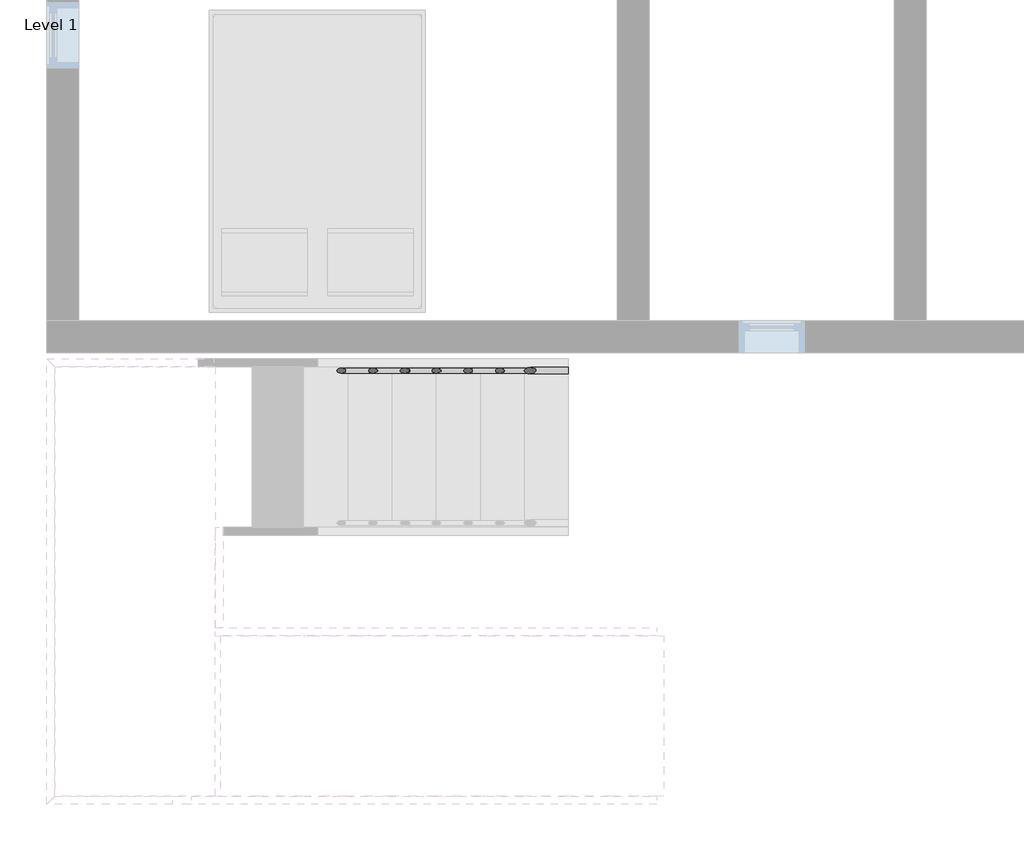
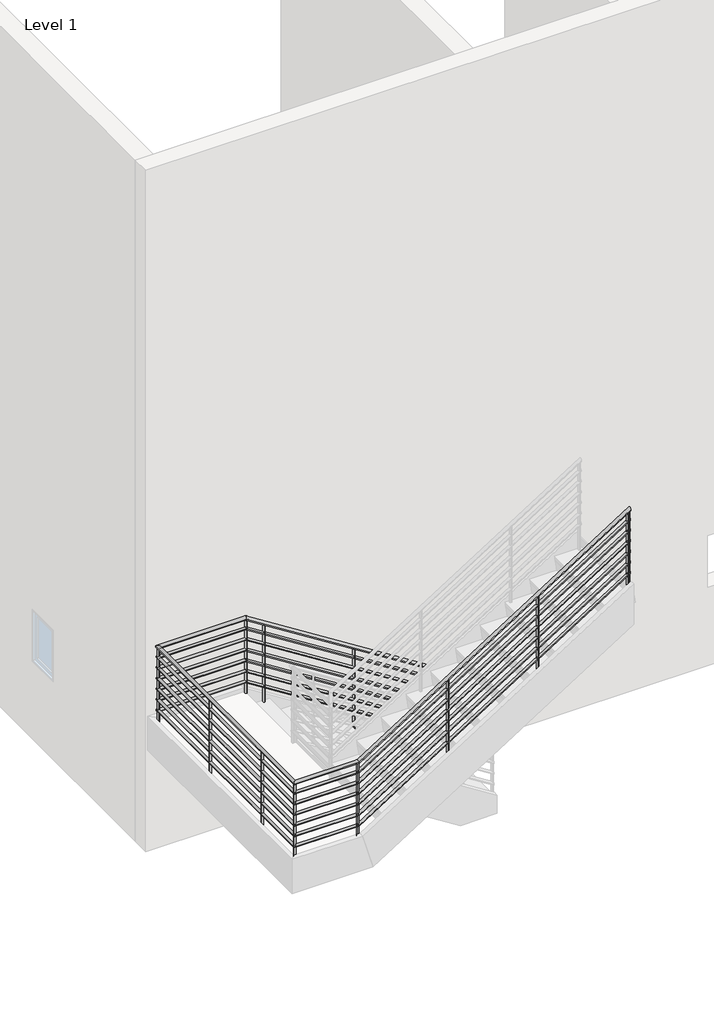
# One storey, part 2 of 4: 1 railing.
"""IFC4 building model written with IfcOpenShell, lengths in millimetres."""

from ifc_helpers import new_model, si_unit, point, frame, frame_2d, origin, place, context, project, spatial, circle_curve, ellipse_curve, trimmed, segment, composite_curve, outline, extrude, element, save
from ifc_brep_helpers import plane_surface, cylinder_surface, advanced_brep

model = new_model("IFC4")

# Units and contexts
model_context = context("Model", 3, world=origin())
ifc_project = project(units=[si_unit("LENGTHUNIT", "METRE", prefix="MILLI")], contexts=[model_context])

# Site, building, storey
site = spatial("IfcSite", under=ifc_project)
building = spatial("IfcBuilding", under=site)
storey = spatial("IfcBuildingStorey", under=building, Name="Level 1", Elevation=0.0)

# Railing
placement = place(None, origin())
element("IfcRailing", 1, ObjectType="900mm Pipe", at=placement, inside=storey, context=model_context, shape_type="SolidModel", body=[
    advanced_brep(
    [(-8274.8492596, 6241.5562283, 1050.2491997), (-8274.8492596, 6201.5562283, 1050.2491997), (-10480.6427126, 6241.5562283, 2445.2173913), (-10480.6427126, 6201.5562283, 2445.2173913), (-11469.4750408, 6241.5562283, 2445.2173913), (-11429.4750408, 6201.5562283, 2445.2173913), (-11469.4750408, 3575.930447, 2445.2173913), (-11429.4750408, 3615.930447, 2445.2173913), (-10744.0558066, 3575.930447, 2445.2173913), (-10744.0558066, 3615.930447, 2445.2173913), (-7724.8492596, 3575.930447, 4354.5970258), (-7724.8492596, 3615.930447, 4354.5970258)],
    [
        (0, 1, ellipse_curve(frame((-8274.8492596, 6221.5562283, 1050.2491997), z_axis=(1.0, 0.0, 0.0), x_axis=(0.0, 0.0, -1.0)), 23.6638438, 20.0)),
        (1, 0, ellipse_curve(frame((-8274.8492596, 6221.5562283, 1050.2491997), z_axis=(1.0, 0.0, 0.0), x_axis=(0.0, 0.0, -1.0)), 23.6638438, 20.0)),
        (0, 2),
        (2, 3, ellipse_curve(frame((-10480.6427126, 6221.5562283, 2445.2173913), z_axis=(0.9605132043335073, 0.0, -0.2782344053149758), x_axis=(-0.2782344053149764, 0.0, -0.9605132043335071)), 20.822202, 20.0)),
        (3, 1),
        (3, 2, ellipse_curve(frame((-10480.6427126, 6221.5562283, 2445.2173913), z_axis=(0.9605132043335073, 0.0, -0.2782344053149758), x_axis=(-0.2782344053149764, 0.0, -0.9605132043335071)), 20.822202, 20.0)),
        (2, 4),
        (4, 5, ellipse_curve(frame((-11449.4750408, 6221.5562283, 2445.2173913), z_axis=(0.7071067811865516, 0.7071067811865435, 0.0), x_axis=(0.7071067811865436, -0.7071067811865516, 0.0)), 28.2842712, 20.0)),
        (5, 3),
        (5, 4, ellipse_curve(frame((-11449.4750408, 6221.5562283, 2445.2173913), z_axis=(0.7071067811865516, 0.7071067811865435, 0.0), x_axis=(0.7071067811865436, -0.7071067811865516, 0.0)), 28.2842712, 20.0)),
        (4, 6),
        (6, 7, ellipse_curve(frame((-11449.4750408, 3595.930447, 2445.2173913), z_axis=(-0.7071067811865436, 0.7071067811865513, 0.0), x_axis=(0.7071067811865512, 0.7071067811865438, 0.0)), 28.2842712, 20.0)),
        (7, 5),
        (7, 6, ellipse_curve(frame((-11449.4750408, 3595.930447, 2445.2173913), z_axis=(-0.7071067811865436, 0.7071067811865513, 0.0), x_axis=(0.7071067811865512, 0.7071067811865438, 0.0)), 28.2842712, 20.0)),
        (6, 8),
        (8, 9, ellipse_curve(frame((-10744.0558066, 3595.930447, 2445.2173913), z_axis=(-0.9605132043335073, 0.0, -0.2782344053149758), x_axis=(-0.2782344053149755, 0.0, 0.9605132043335073)), 20.822202, 20.0)),
        (9, 7),
        (9, 8, ellipse_curve(frame((-10744.0558066, 3595.930447, 2445.2173913), z_axis=(-0.9605132043335073, 0.0, -0.2782344053149758), x_axis=(-0.2782344053149755, 0.0, 0.9605132043335073)), 20.822202, 20.0)),
        (10, 11, ellipse_curve(frame((-7724.8492596, 3595.930447, 4354.5970258), z_axis=(1.0, 0.0, 0.0), x_axis=(0.0, 0.0, -1.0)), 23.6638438, 20.0)),
        (11, 10, ellipse_curve(frame((-7724.8492596, 3595.930447, 4354.5970258), z_axis=(1.0, 0.0, 0.0), x_axis=(0.0, 0.0, -1.0)), 23.6638438, 20.0)),
        (8, 10),
        (11, 9),
    ],
    [
        plane_surface(frame((-8274.8492596, 6221.5562283, 1073.9130435), z_axis=(1.0, 0.0, 0.0), x_axis=(0.0, -1.0, 0.0))),
        cylinder_surface(frame((-8285.5391724, 6221.5562283, 1057.0096189), z_axis=(0.8451712313980436, 0.0, -0.5344956404098303), x_axis=(0.0, -1.0, 0.0)), 20.0),
        cylinder_surface(frame((-10474.8492596, 6221.5562283, 2445.2173913), z_axis=(1.0, 0.0, 0.0), x_axis=(0.0, -1.0, 0.0)), 20.0),
        cylinder_surface(frame((-11449.4750408, 6221.5562283, 2445.2173913), z_axis=(0.0, 1.0, 0.0), x_axis=(1.0, 0.0, 0.0)), 20.0),
        cylinder_surface(frame((-11449.4750408, 3595.930447, 2445.2173913), z_axis=(-1.0, 0.0, 0.0), x_axis=(0.0, 1.0, 0.0)), 20.0),
        plane_surface(frame((-7724.8492596, 3595.930447, 4378.2608696), z_axis=(1.0, 0.0, 0.0), x_axis=(0.0, 1.0, 0.0))),
        cylinder_surface(frame((-10739.1593468, 3595.930447, 2448.3139667), z_axis=(-0.8451712313980436, 0.0, -0.5344956404098303), x_axis=(0.0, 1.0, 0.0)), 20.0),
    ],
    [
        (0, [[1, 2]]),
        (1, [[-1, 3, 4, 5]]),
        (1, [[-2, -5, 6, -3]]),
        (2, [[-4, 7, 8, 9]]),
        (2, [[-6, -9, 10, -7]]),
        (3, [[-8, 11, 12, 13]]),
        (3, [[-10, -13, 14, -11]]),
        (4, [[-12, 15, 16, 17]]),
        (4, [[-14, -17, 18, -15]]),
        (5, [[19, 20]]),
        (6, [[-16, 21, -20, 22]]),
        (6, [[-18, -22, -19, -21]]),
    ],
),
    advanced_brep(
    [(-8274.8492596, 6206.5562283, 931.1651606), (-8274.8492596, 6236.5562283, 931.1651606), (-10479.1943493, 6206.5562283, 2325.2173913), (-10479.1943493, 6236.5562283, 2325.2173913), (-11434.4750408, 6206.5562283, 2325.2173913), (-11464.4750408, 6236.5562283, 2325.2173913), (-11434.4750408, 3610.930447, 2325.2173913), (-11464.4750408, 3580.930447, 2325.2173913), (-10745.5041698, 3610.930447, 2325.2173913), (-10745.5041698, 3580.930447, 2325.2173913), (-7724.8492596, 3610.930447, 4235.5129867), (-7724.8492596, 3580.930447, 4235.5129867)],
    [
        (0, 1, ellipse_curve(frame((-8274.8492596, 6221.5562283, 931.1651606), z_axis=(1.0, 0.0, 0.0), x_axis=(0.0, 0.0, -1.0)), 17.7478828, 15.0)),
        (1, 0, ellipse_curve(frame((-8274.8492596, 6221.5562283, 931.1651606), z_axis=(1.0, 0.0, 0.0), x_axis=(0.0, 0.0, -1.0)), 17.7478828, 15.0)),
        (0, 2),
        (2, 3, ellipse_curve(frame((-10479.1943493, 6221.5562283, 2325.2173913), z_axis=(0.9605132043335073, 0.0, -0.2782344053149758), x_axis=(-0.2782344053149764, 0.0, -0.9605132043335071)), 15.6166515, 15.0)),
        (3, 1),
        (3, 2, ellipse_curve(frame((-10479.1943493, 6221.5562283, 2325.2173913), z_axis=(0.9605132043335073, 0.0, -0.2782344053149758), x_axis=(-0.2782344053149764, 0.0, -0.9605132043335071)), 15.6166515, 15.0)),
        (2, 4),
        (4, 5, ellipse_curve(frame((-11449.4750408, 6221.5562283, 2325.2173913), z_axis=(0.7071067811865516, 0.7071067811865435, 0.0), x_axis=(0.7071067811865436, -0.7071067811865516, 0.0)), 21.2132034, 15.0)),
        (5, 3),
        (5, 4, ellipse_curve(frame((-11449.4750408, 6221.5562283, 2325.2173913), z_axis=(0.7071067811865516, 0.7071067811865435, 0.0), x_axis=(0.7071067811865436, -0.7071067811865516, 0.0)), 21.2132034, 15.0)),
        (4, 6),
        (6, 7, ellipse_curve(frame((-11449.4750408, 3595.930447, 2325.2173913), z_axis=(-0.7071067811865436, 0.7071067811865513, 0.0), x_axis=(0.7071067811865512, 0.7071067811865438, 0.0)), 21.2132034, 15.0)),
        (7, 5),
        (7, 6, ellipse_curve(frame((-11449.4750408, 3595.930447, 2325.2173913), z_axis=(-0.7071067811865436, 0.7071067811865513, 0.0), x_axis=(0.7071067811865512, 0.7071067811865438, 0.0)), 21.2132034, 15.0)),
        (6, 8),
        (8, 9, ellipse_curve(frame((-10745.5041698, 3595.930447, 2325.2173913), z_axis=(-0.9605132043335072, 0.0, -0.27823440531497556), x_axis=(-0.2782344053149761, 0.0, 0.9605132043335072)), 15.6166515, 15.0)),
        (9, 7),
        (9, 8, ellipse_curve(frame((-10745.5041698, 3595.930447, 2325.2173913), z_axis=(-0.9605132043335072, 0.0, -0.27823440531497556), x_axis=(-0.2782344053149761, 0.0, 0.9605132043335072)), 15.6166515, 15.0)),
        (10, 11, ellipse_curve(frame((-7724.8492596, 3595.930447, 4235.5129867), z_axis=(1.0, 0.0, 0.0), x_axis=(0.0, 0.0, -1.0)), 17.7478828, 15.0)),
        (11, 10, ellipse_curve(frame((-7724.8492596, 3595.930447, 4235.5129867), z_axis=(1.0, 0.0, 0.0), x_axis=(0.0, 0.0, -1.0)), 17.7478828, 15.0)),
        (8, 10),
        (11, 9),
    ],
    [
        plane_surface(frame((-8274.8492596, 6221.5562283, 948.9130435), z_axis=(1.0, 0.0, 0.0), x_axis=(0.0, -1.0, 0.0))),
        cylinder_surface(frame((-8282.8666942, 6221.5562283, 936.235475), z_axis=(0.8451712313980436, 0.0, -0.5344956404098303), x_axis=(0.0, 1.0, 0.0)), 15.0),
        cylinder_surface(frame((-10474.8492596, 6221.5562283, 2325.2173913), z_axis=(1.0, 0.0, 0.0), x_axis=(0.0, 1.0, 0.0)), 15.0),
        cylinder_surface(frame((-11449.4750408, 6221.5562283, 2325.2173913), z_axis=(0.0, 1.0, 0.0), x_axis=(-1.0, 0.0, 0.0)), 15.0),
        cylinder_surface(frame((-11449.4750408, 3595.930447, 2325.2173913), z_axis=(-1.0, 0.0, 0.0), x_axis=(0.0, -1.0, 0.0)), 15.0),
        plane_surface(frame((-7724.8492596, 3595.930447, 4253.2608696), z_axis=(1.0, 0.0, 0.0), x_axis=(0.0, 1.0, 0.0))),
        cylinder_surface(frame((-10741.831825, 3595.930447, 2327.5398228), z_axis=(-0.8451712313980437, 0.0, -0.5344956404098301), x_axis=(0.0, -1.0, 0.0)), 15.0),
    ],
    [
        (0, [[1, 2]]),
        (1, [[-1, 3, 4, 5]]),
        (1, [[-2, -5, 6, -3]]),
        (2, [[-4, 7, 8, 9]]),
        (2, [[-6, -9, 10, -7]]),
        (3, [[-8, 11, 12, 13]]),
        (3, [[-10, -13, 14, -11]]),
        (4, [[-12, 15, 16, 17]]),
        (4, [[-14, -17, 18, -15]]),
        (5, [[19, 20]]),
        (6, [[-16, 21, -20, 22]]),
        (6, [[-18, -22, -19, -21]]),
    ],
),
    advanced_brep(
    [(-8274.8492596, 6206.5562283, 806.1651606), (-8274.8492596, 6236.5562283, 806.1651606), (-10479.1943493, 6206.5562283, 2200.2173913), (-10479.1943493, 6236.5562283, 2200.2173913), (-11434.4750408, 6206.5562283, 2200.2173913), (-11464.4750408, 6236.5562283, 2200.2173913), (-11434.4750408, 3610.930447, 2200.2173913), (-11464.4750408, 3580.930447, 2200.2173913), (-10745.5041698, 3610.930447, 2200.2173913), (-10745.5041698, 3580.930447, 2200.2173913), (-7724.8492596, 3610.930447, 4110.5129867), (-7724.8492596, 3580.930447, 4110.5129867)],
    [
        (0, 1, ellipse_curve(frame((-8274.8492596, 6221.5562283, 806.1651606), z_axis=(1.0, 0.0, 0.0), x_axis=(0.0, 0.0, -1.0)), 17.7478828, 15.0)),
        (1, 0, ellipse_curve(frame((-8274.8492596, 6221.5562283, 806.1651606), z_axis=(1.0, 0.0, 0.0), x_axis=(0.0, 0.0, -1.0)), 17.7478828, 15.0)),
        (0, 2),
        (2, 3, ellipse_curve(frame((-10479.1943493, 6221.5562283, 2200.2173913), z_axis=(0.9605132043335073, 0.0, -0.2782344053149758), x_axis=(-0.2782344053149764, 0.0, -0.9605132043335071)), 15.6166515, 15.0)),
        (3, 1),
        (3, 2, ellipse_curve(frame((-10479.1943493, 6221.5562283, 2200.2173913), z_axis=(0.9605132043335073, 0.0, -0.2782344053149758), x_axis=(-0.2782344053149764, 0.0, -0.9605132043335071)), 15.6166515, 15.0)),
        (2, 4),
        (4, 5, ellipse_curve(frame((-11449.4750408, 6221.5562283, 2200.2173913), z_axis=(0.7071067811865516, 0.7071067811865435, 0.0), x_axis=(0.7071067811865436, -0.7071067811865516, 0.0)), 21.2132034, 15.0)),
        (5, 3),
        (5, 4, ellipse_curve(frame((-11449.4750408, 6221.5562283, 2200.2173913), z_axis=(0.7071067811865516, 0.7071067811865435, 0.0), x_axis=(0.7071067811865436, -0.7071067811865516, 0.0)), 21.2132034, 15.0)),
        (4, 6),
        (6, 7, ellipse_curve(frame((-11449.4750408, 3595.930447, 2200.2173913), z_axis=(-0.7071067811865436, 0.7071067811865513, 0.0), x_axis=(0.7071067811865512, 0.7071067811865438, 0.0)), 21.2132034, 15.0)),
        (7, 5),
        (7, 6, ellipse_curve(frame((-11449.4750408, 3595.930447, 2200.2173913), z_axis=(-0.7071067811865436, 0.7071067811865513, 0.0), x_axis=(0.7071067811865512, 0.7071067811865438, 0.0)), 21.2132034, 15.0)),
        (6, 8),
        (8, 9, ellipse_curve(frame((-10745.5041698, 3595.930447, 2200.2173913), z_axis=(-0.9605132043335072, 0.0, -0.2782344053149756), x_axis=(-0.27823440531497606, 0.0, 0.9605132043335073)), 15.6166515, 15.0)),
        (9, 7),
        (9, 8, ellipse_curve(frame((-10745.5041698, 3595.930447, 2200.2173913), z_axis=(-0.9605132043335072, 0.0, -0.2782344053149756), x_axis=(-0.27823440531497606, 0.0, 0.9605132043335073)), 15.6166515, 15.0)),
        (10, 11, ellipse_curve(frame((-7724.8492596, 3595.930447, 4110.5129867), z_axis=(1.0, 0.0, 0.0), x_axis=(0.0, 0.0, -1.0)), 17.7478828, 15.0)),
        (11, 10, ellipse_curve(frame((-7724.8492596, 3595.930447, 4110.5129867), z_axis=(1.0, 0.0, 0.0), x_axis=(0.0, 0.0, -1.0)), 17.7478828, 15.0)),
        (8, 10),
        (11, 9),
    ],
    [
        plane_surface(frame((-8274.8492596, 6221.5562283, 823.9130435), z_axis=(1.0, 0.0, 0.0), x_axis=(0.0, -1.0, 0.0))),
        cylinder_surface(frame((-8282.8666942, 6221.5562283, 811.235475), z_axis=(0.8451712313980436, 0.0, -0.5344956404098303), x_axis=(0.0, 1.0, 0.0)), 15.0),
        cylinder_surface(frame((-10474.8492596, 6221.5562283, 2200.2173913), z_axis=(1.0, 0.0, 0.0), x_axis=(0.0, 1.0, 0.0)), 15.0),
        cylinder_surface(frame((-11449.4750408, 6221.5562283, 2200.2173913), z_axis=(0.0, 1.0, 0.0), x_axis=(-1.0, 0.0, 0.0)), 15.0),
        cylinder_surface(frame((-11449.4750408, 3595.930447, 2200.2173913), z_axis=(-1.0, 0.0, 0.0), x_axis=(0.0, -1.0, 0.0)), 15.0),
        plane_surface(frame((-7724.8492596, 3595.930447, 4128.2608696), z_axis=(1.0, 0.0, 0.0), x_axis=(0.0, 1.0, 0.0))),
        cylinder_surface(frame((-10741.831825, 3595.930447, 2202.5398228), z_axis=(-0.8451712313980437, 0.0, -0.5344956404098302), x_axis=(0.0, -1.0, 0.0)), 15.0),
    ],
    [
        (0, [[1, 2]]),
        (1, [[-1, 3, 4, 5]]),
        (1, [[-2, -5, 6, -3]]),
        (2, [[-4, 7, 8, 9]]),
        (2, [[-6, -9, 10, -7]]),
        (3, [[-8, 11, 12, 13]]),
        (3, [[-10, -13, 14, -11]]),
        (4, [[-12, 15, 16, 17]]),
        (4, [[-14, -17, 18, -15]]),
        (5, [[19, 20]]),
        (6, [[-16, 21, -20, 22]]),
        (6, [[-18, -22, -19, -21]]),
    ],
),
    advanced_brep(
    [(-8274.8492596, 6206.5562283, 681.1651606), (-8274.8492596, 6236.5562283, 681.1651606), (-10479.1943493, 6206.5562283, 2075.2173913), (-10479.1943493, 6236.5562283, 2075.2173913), (-11434.4750408, 6206.5562283, 2075.2173913), (-11464.4750408, 6236.5562283, 2075.2173913), (-11434.4750408, 3610.930447, 2075.2173913), (-11464.4750408, 3580.930447, 2075.2173913), (-10745.5041698, 3610.930447, 2075.2173913), (-10745.5041698, 3580.930447, 2075.2173913), (-7724.8492596, 3610.930447, 3985.5129867), (-7724.8492596, 3580.930447, 3985.5129867)],
    [
        (0, 1, ellipse_curve(frame((-8274.8492596, 6221.5562283, 681.1651606), z_axis=(1.0, 0.0, 0.0), x_axis=(0.0, 0.0, -1.0)), 17.7478828, 15.0)),
        (1, 0, ellipse_curve(frame((-8274.8492596, 6221.5562283, 681.1651606), z_axis=(1.0, 0.0, 0.0), x_axis=(0.0, 0.0, -1.0)), 17.7478828, 15.0)),
        (0, 2),
        (2, 3, ellipse_curve(frame((-10479.1943493, 6221.5562283, 2075.2173913), z_axis=(0.9605132043335073, 0.0, -0.2782344053149758), x_axis=(-0.2782344053149764, 0.0, -0.9605132043335071)), 15.6166515, 15.0)),
        (3, 1),
        (3, 2, ellipse_curve(frame((-10479.1943493, 6221.5562283, 2075.2173913), z_axis=(0.9605132043335073, 0.0, -0.2782344053149758), x_axis=(-0.2782344053149764, 0.0, -0.9605132043335071)), 15.6166515, 15.0)),
        (2, 4),
        (4, 5, ellipse_curve(frame((-11449.4750408, 6221.5562283, 2075.2173913), z_axis=(0.7071067811865516, 0.7071067811865435, 0.0), x_axis=(0.7071067811865436, -0.7071067811865516, 0.0)), 21.2132034, 15.0)),
        (5, 3),
        (5, 4, ellipse_curve(frame((-11449.4750408, 6221.5562283, 2075.2173913), z_axis=(0.7071067811865516, 0.7071067811865435, 0.0), x_axis=(0.7071067811865436, -0.7071067811865516, 0.0)), 21.2132034, 15.0)),
        (4, 6),
        (6, 7, ellipse_curve(frame((-11449.4750408, 3595.930447, 2075.2173913), z_axis=(-0.7071067811865436, 0.7071067811865513, 0.0), x_axis=(0.7071067811865512, 0.7071067811865438, 0.0)), 21.2132034, 15.0)),
        (7, 5),
        (7, 6, ellipse_curve(frame((-11449.4750408, 3595.930447, 2075.2173913), z_axis=(-0.7071067811865436, 0.7071067811865513, 0.0), x_axis=(0.7071067811865512, 0.7071067811865438, 0.0)), 21.2132034, 15.0)),
        (6, 8),
        (8, 9, ellipse_curve(frame((-10745.5041698, 3595.930447, 2075.2173913), z_axis=(-0.9605132043335073, 0.0, -0.2782344053149758), x_axis=(-0.2782344053149755, 0.0, 0.9605132043335073)), 15.6166515, 15.0)),
        (9, 7),
        (9, 8, ellipse_curve(frame((-10745.5041698, 3595.930447, 2075.2173913), z_axis=(-0.9605132043335073, 0.0, -0.2782344053149758), x_axis=(-0.2782344053149755, 0.0, 0.9605132043335073)), 15.6166515, 15.0)),
        (10, 11, ellipse_curve(frame((-7724.8492596, 3595.930447, 3985.5129867), z_axis=(1.0, 0.0, 0.0), x_axis=(0.0, 0.0, -1.0)), 17.7478828, 15.0)),
        (11, 10, ellipse_curve(frame((-7724.8492596, 3595.930447, 3985.5129867), z_axis=(1.0, 0.0, 0.0), x_axis=(0.0, 0.0, -1.0)), 17.7478828, 15.0)),
        (8, 10),
        (11, 9),
    ],
    [
        plane_surface(frame((-8274.8492596, 6221.5562283, 698.9130435), z_axis=(1.0, 0.0, 0.0), x_axis=(0.0, -1.0, 0.0))),
        cylinder_surface(frame((-8282.8666942, 6221.5562283, 686.235475), z_axis=(0.8451712313980436, 0.0, -0.5344956404098303), x_axis=(0.0, 1.0, 0.0)), 15.0),
        cylinder_surface(frame((-10474.8492596, 6221.5562283, 2075.2173913), z_axis=(1.0, 0.0, 0.0), x_axis=(0.0, 1.0, 0.0)), 15.0),
        cylinder_surface(frame((-11449.4750408, 6221.5562283, 2075.2173913), z_axis=(0.0, 1.0, 0.0), x_axis=(-1.0, 0.0, 0.0)), 15.0),
        cylinder_surface(frame((-11449.4750408, 3595.930447, 2075.2173913), z_axis=(-1.0, 0.0, 0.0), x_axis=(0.0, -1.0, 0.0)), 15.0),
        plane_surface(frame((-7724.8492596, 3595.930447, 4003.2608696), z_axis=(1.0, 0.0, 0.0), x_axis=(0.0, 1.0, 0.0))),
        cylinder_surface(frame((-10741.831825, 3595.930447, 2077.5398228), z_axis=(-0.8451712313980436, 0.0, -0.5344956404098303), x_axis=(0.0, -1.0, 0.0)), 15.0),
    ],
    [
        (0, [[1, 2]]),
        (1, [[-1, 3, 4, 5]]),
        (1, [[-2, -5, 6, -3]]),
        (2, [[-4, 7, 8, 9]]),
        (2, [[-6, -9, 10, -7]]),
        (3, [[-8, 11, 12, 13]]),
        (3, [[-10, -13, 14, -11]]),
        (4, [[-12, 15, 16, 17]]),
        (4, [[-14, -17, 18, -15]]),
        (5, [[19, 20]]),
        (6, [[-16, 21, -20, 22]]),
        (6, [[-18, -22, -19, -21]]),
    ],
),
    advanced_brep(
    [(-8274.8492596, 6206.5562283, 556.1651606), (-8274.8492596, 6236.5562283, 556.1651606), (-10479.1943493, 6206.5562283, 1950.2173913), (-10479.1943493, 6236.5562283, 1950.2173913), (-11434.4750408, 6206.5562283, 1950.2173913), (-11464.4750408, 6236.5562283, 1950.2173913), (-11434.4750408, 3610.930447, 1950.2173913), (-11464.4750408, 3580.930447, 1950.2173913), (-10745.5041698, 3610.930447, 1950.2173913), (-10745.5041698, 3580.930447, 1950.2173913), (-7724.8492596, 3610.930447, 3860.5129867), (-7724.8492596, 3580.930447, 3860.5129867)],
    [
        (0, 1, ellipse_curve(frame((-8274.8492596, 6221.5562283, 556.1651606), z_axis=(1.0, 0.0, 0.0), x_axis=(0.0, 0.0, -1.0)), 17.7478828, 15.0)),
        (1, 0, ellipse_curve(frame((-8274.8492596, 6221.5562283, 556.1651606), z_axis=(1.0, 0.0, 0.0), x_axis=(0.0, 0.0, -1.0)), 17.7478828, 15.0)),
        (0, 2),
        (2, 3, ellipse_curve(frame((-10479.1943493, 6221.5562283, 1950.2173913), z_axis=(0.9605132043335073, 0.0, -0.2782344053149758), x_axis=(-0.2782344053149764, 0.0, -0.9605132043335071)), 15.6166515, 15.0)),
        (3, 1),
        (3, 2, ellipse_curve(frame((-10479.1943493, 6221.5562283, 1950.2173913), z_axis=(0.9605132043335073, 0.0, -0.2782344053149758), x_axis=(-0.2782344053149764, 0.0, -0.9605132043335071)), 15.6166515, 15.0)),
        (2, 4),
        (4, 5, ellipse_curve(frame((-11449.4750408, 6221.5562283, 1950.2173913), z_axis=(0.7071067811865516, 0.7071067811865435, 0.0), x_axis=(0.7071067811865436, -0.7071067811865516, 0.0)), 21.2132034, 15.0)),
        (5, 3),
        (5, 4, ellipse_curve(frame((-11449.4750408, 6221.5562283, 1950.2173913), z_axis=(0.7071067811865516, 0.7071067811865435, 0.0), x_axis=(0.7071067811865436, -0.7071067811865516, 0.0)), 21.2132034, 15.0)),
        (4, 6),
        (6, 7, ellipse_curve(frame((-11449.4750408, 3595.930447, 1950.2173913), z_axis=(-0.7071067811865436, 0.7071067811865513, 0.0), x_axis=(0.7071067811865512, 0.7071067811865438, 0.0)), 21.2132034, 15.0)),
        (7, 5),
        (7, 6, ellipse_curve(frame((-11449.4750408, 3595.930447, 1950.2173913), z_axis=(-0.7071067811865436, 0.7071067811865513, 0.0), x_axis=(0.7071067811865512, 0.7071067811865438, 0.0)), 21.2132034, 15.0)),
        (6, 8),
        (8, 9, ellipse_curve(frame((-10745.5041698, 3595.930447, 1950.2173913), z_axis=(-0.9605132043335072, 0.0, -0.2782344053149756), x_axis=(-0.27823440531497606, 0.0, 0.9605132043335073)), 15.6166515, 15.0)),
        (9, 7),
        (9, 8, ellipse_curve(frame((-10745.5041698, 3595.930447, 1950.2173913), z_axis=(-0.9605132043335072, 0.0, -0.2782344053149756), x_axis=(-0.27823440531497606, 0.0, 0.9605132043335073)), 15.6166515, 15.0)),
        (10, 11, ellipse_curve(frame((-7724.8492596, 3595.930447, 3860.5129867), z_axis=(1.0, 0.0, 0.0), x_axis=(0.0, 0.0, -1.0)), 17.7478828, 15.0)),
        (11, 10, ellipse_curve(frame((-7724.8492596, 3595.930447, 3860.5129867), z_axis=(1.0, 0.0, 0.0), x_axis=(0.0, 0.0, -1.0)), 17.7478828, 15.0)),
        (8, 10),
        (11, 9),
    ],
    [
        plane_surface(frame((-8274.8492596, 6221.5562283, 573.9130435), z_axis=(1.0, 0.0, 0.0), x_axis=(0.0, -1.0, 0.0))),
        cylinder_surface(frame((-8282.8666942, 6221.5562283, 561.235475), z_axis=(0.8451712313980436, 0.0, -0.5344956404098303), x_axis=(0.0, 1.0, 0.0)), 15.0),
        cylinder_surface(frame((-10474.8492596, 6221.5562283, 1950.2173913), z_axis=(1.0, 0.0, 0.0), x_axis=(0.0, 1.0, 0.0)), 15.0),
        cylinder_surface(frame((-11449.4750408, 6221.5562283, 1950.2173913), z_axis=(0.0, 1.0, 0.0), x_axis=(-1.0, 0.0, 0.0)), 15.0),
        cylinder_surface(frame((-11449.4750408, 3595.930447, 1950.2173913), z_axis=(-1.0, 0.0, 0.0), x_axis=(0.0, -1.0, 0.0)), 15.0),
        plane_surface(frame((-7724.8492596, 3595.930447, 3878.2608696), z_axis=(1.0, 0.0, 0.0), x_axis=(0.0, 1.0, 0.0))),
        cylinder_surface(frame((-10741.831825, 3595.930447, 1952.5398228), z_axis=(-0.8451712313980437, 0.0, -0.5344956404098302), x_axis=(0.0, -1.0, 0.0)), 15.0),
    ],
    [
        (0, [[1, 2]]),
        (1, [[-1, 3, 4, 5]]),
        (1, [[-2, -5, 6, -3]]),
        (2, [[-4, 7, 8, 9]]),
        (2, [[-6, -9, 10, -7]]),
        (3, [[-8, 11, 12, 13]]),
        (3, [[-10, -13, 14, -11]]),
        (4, [[-12, 15, 16, 17]]),
        (4, [[-14, -17, 18, -15]]),
        (5, [[19, 20]]),
        (6, [[-16, 21, -20, 22]]),
        (6, [[-18, -22, -19, -21]]),
    ],
),
    advanced_brep(
    [(-8274.8492596, 6206.5562283, 431.1651606), (-8274.8492596, 6236.5562283, 431.1651606), (-10479.1943493, 6206.5562283, 1825.2173913), (-10479.1943493, 6236.5562283, 1825.2173913), (-11434.4750408, 6206.5562283, 1825.2173913), (-11464.4750408, 6236.5562283, 1825.2173913), (-11434.4750408, 3610.930447, 1825.2173913), (-11464.4750408, 3580.930447, 1825.2173913), (-10745.5041698, 3610.930447, 1825.2173913), (-10745.5041698, 3580.930447, 1825.2173913), (-7724.8492596, 3610.930447, 3735.5129867), (-7724.8492596, 3580.930447, 3735.5129867)],
    [
        (0, 1, ellipse_curve(frame((-8274.8492596, 6221.5562283, 431.1651606), z_axis=(1.0, 0.0, 0.0), x_axis=(0.0, 0.0, -1.0)), 17.7478828, 15.0)),
        (1, 0, ellipse_curve(frame((-8274.8492596, 6221.5562283, 431.1651606), z_axis=(1.0, 0.0, 0.0), x_axis=(0.0, 0.0, -1.0)), 17.7478828, 15.0)),
        (0, 2),
        (2, 3, ellipse_curve(frame((-10479.1943493, 6221.5562283, 1825.2173913), z_axis=(0.9605132043335073, 0.0, -0.2782344053149758), x_axis=(-0.2782344053149764, 0.0, -0.9605132043335071)), 15.6166515, 15.0)),
        (3, 1),
        (3, 2, ellipse_curve(frame((-10479.1943493, 6221.5562283, 1825.2173913), z_axis=(0.9605132043335073, 0.0, -0.2782344053149758), x_axis=(-0.2782344053149764, 0.0, -0.9605132043335071)), 15.6166515, 15.0)),
        (2, 4),
        (4, 5, ellipse_curve(frame((-11449.4750408, 6221.5562283, 1825.2173913), z_axis=(0.7071067811865516, 0.7071067811865435, 0.0), x_axis=(0.7071067811865436, -0.7071067811865516, 0.0)), 21.2132034, 15.0)),
        (5, 3),
        (5, 4, ellipse_curve(frame((-11449.4750408, 6221.5562283, 1825.2173913), z_axis=(0.7071067811865516, 0.7071067811865435, 0.0), x_axis=(0.7071067811865436, -0.7071067811865516, 0.0)), 21.2132034, 15.0)),
        (4, 6),
        (6, 7, ellipse_curve(frame((-11449.4750408, 3595.930447, 1825.2173913), z_axis=(-0.7071067811865436, 0.7071067811865513, 0.0), x_axis=(0.7071067811865512, 0.7071067811865438, 0.0)), 21.2132034, 15.0)),
        (7, 5),
        (7, 6, ellipse_curve(frame((-11449.4750408, 3595.930447, 1825.2173913), z_axis=(-0.7071067811865436, 0.7071067811865513, 0.0), x_axis=(0.7071067811865512, 0.7071067811865438, 0.0)), 21.2132034, 15.0)),
        (6, 8),
        (8, 9, ellipse_curve(frame((-10745.5041698, 3595.930447, 1825.2173913), z_axis=(-0.9605132043335072, 0.0, -0.27823440531497556), x_axis=(-0.2782344053149761, 0.0, 0.9605132043335072)), 15.6166515, 15.0)),
        (9, 7),
        (9, 8, ellipse_curve(frame((-10745.5041698, 3595.930447, 1825.2173913), z_axis=(-0.9605132043335072, 0.0, -0.27823440531497556), x_axis=(-0.2782344053149761, 0.0, 0.9605132043335072)), 15.6166515, 15.0)),
        (10, 11, ellipse_curve(frame((-7724.8492596, 3595.930447, 3735.5129867), z_axis=(1.0, 0.0, 0.0), x_axis=(0.0, 0.0, -1.0)), 17.7478828, 15.0)),
        (11, 10, ellipse_curve(frame((-7724.8492596, 3595.930447, 3735.5129867), z_axis=(1.0, 0.0, 0.0), x_axis=(0.0, 0.0, -1.0)), 17.7478828, 15.0)),
        (8, 10),
        (11, 9),
    ],
    [
        plane_surface(frame((-8274.8492596, 6221.5562283, 448.9130435), z_axis=(1.0, 0.0, 0.0), x_axis=(0.0, -1.0, 0.0))),
        cylinder_surface(frame((-8282.8666942, 6221.5562283, 436.235475), z_axis=(0.8451712313980436, 0.0, -0.5344956404098303), x_axis=(0.0, 1.0, 0.0)), 15.0),
        cylinder_surface(frame((-10474.8492596, 6221.5562283, 1825.2173913), z_axis=(1.0, 0.0, 0.0), x_axis=(0.0, 1.0, 0.0)), 15.0),
        cylinder_surface(frame((-11449.4750408, 6221.5562283, 1825.2173913), z_axis=(0.0, 1.0, 0.0), x_axis=(-1.0, 0.0, 0.0)), 15.0),
        cylinder_surface(frame((-11449.4750408, 3595.930447, 1825.2173913), z_axis=(-1.0, 0.0, 0.0), x_axis=(0.0, -1.0, 0.0)), 15.0),
        plane_surface(frame((-7724.8492596, 3595.930447, 3753.2608696), z_axis=(1.0, 0.0, 0.0), x_axis=(0.0, 1.0, 0.0))),
        cylinder_surface(frame((-10741.831825, 3595.930447, 1827.5398228), z_axis=(-0.8451712313980437, 0.0, -0.5344956404098301), x_axis=(0.0, -1.0, 0.0)), 15.0),
    ],
    [
        (0, [[1, 2]]),
        (1, [[-1, 3, 4, 5]]),
        (1, [[-2, -5, 6, -3]]),
        (2, [[-4, 7, 8, 9]]),
        (2, [[-6, -9, 10, -7]]),
        (3, [[-8, 11, 12, 13]]),
        (3, [[-10, -13, 14, -11]]),
        (4, [[-12, 15, 16, 17]]),
        (4, [[-14, -17, 18, -15]]),
        (5, [[19, 20]]),
        (6, [[-16, 21, -20, 22]]),
        (6, [[-18, -22, -19, -21]]),
    ],
),
    advanced_brep(
    [(-8274.8492596, 6206.5562283, 306.1651606), (-8274.8492596, 6236.5562283, 306.1651606), (-10479.1943493, 6206.5562283, 1700.2173913), (-10479.1943493, 6236.5562283, 1700.2173913), (-11434.4750408, 6206.5562283, 1700.2173913), (-11464.4750408, 6236.5562283, 1700.2173913), (-11434.4750408, 3610.930447, 1700.2173913), (-11464.4750408, 3580.930447, 1700.2173913), (-10745.5041698, 3610.930447, 1700.2173913), (-10745.5041698, 3580.930447, 1700.2173913), (-7724.8492596, 3610.930447, 3610.5129867), (-7724.8492596, 3580.930447, 3610.5129867)],
    [
        (0, 1, ellipse_curve(frame((-8274.8492596, 6221.5562283, 306.1651606), z_axis=(1.0, 0.0, 0.0), x_axis=(0.0, 0.0, -1.0)), 17.7478828, 15.0)),
        (1, 0, ellipse_curve(frame((-8274.8492596, 6221.5562283, 306.1651606), z_axis=(1.0, 0.0, 0.0), x_axis=(0.0, 0.0, -1.0)), 17.7478828, 15.0)),
        (0, 2),
        (2, 3, ellipse_curve(frame((-10479.1943493, 6221.5562283, 1700.2173913), z_axis=(0.9605132043335073, 0.0, -0.2782344053149758), x_axis=(-0.2782344053149764, 0.0, -0.9605132043335071)), 15.6166515, 15.0)),
        (3, 1),
        (3, 2, ellipse_curve(frame((-10479.1943493, 6221.5562283, 1700.2173913), z_axis=(0.9605132043335073, 0.0, -0.2782344053149758), x_axis=(-0.2782344053149764, 0.0, -0.9605132043335071)), 15.6166515, 15.0)),
        (2, 4),
        (4, 5, ellipse_curve(frame((-11449.4750408, 6221.5562283, 1700.2173913), z_axis=(0.7071067811865516, 0.7071067811865435, 0.0), x_axis=(0.7071067811865436, -0.7071067811865516, 0.0)), 21.2132034, 15.0)),
        (5, 3),
        (5, 4, ellipse_curve(frame((-11449.4750408, 6221.5562283, 1700.2173913), z_axis=(0.7071067811865516, 0.7071067811865435, 0.0), x_axis=(0.7071067811865436, -0.7071067811865516, 0.0)), 21.2132034, 15.0)),
        (4, 6),
        (6, 7, ellipse_curve(frame((-11449.4750408, 3595.930447, 1700.2173913), z_axis=(-0.7071067811865436, 0.7071067811865513, 0.0), x_axis=(0.7071067811865512, 0.7071067811865438, 0.0)), 21.2132034, 15.0)),
        (7, 5),
        (7, 6, ellipse_curve(frame((-11449.4750408, 3595.930447, 1700.2173913), z_axis=(-0.7071067811865436, 0.7071067811865513, 0.0), x_axis=(0.7071067811865512, 0.7071067811865438, 0.0)), 21.2132034, 15.0)),
        (6, 8),
        (8, 9, ellipse_curve(frame((-10745.5041698, 3595.930447, 1700.2173913), z_axis=(-0.9605132043335072, 0.0, -0.2782344053149756), x_axis=(-0.27823440531497606, 0.0, 0.9605132043335073)), 15.6166515, 15.0)),
        (9, 7),
        (9, 8, ellipse_curve(frame((-10745.5041698, 3595.930447, 1700.2173913), z_axis=(-0.9605132043335072, 0.0, -0.2782344053149756), x_axis=(-0.27823440531497606, 0.0, 0.9605132043335073)), 15.6166515, 15.0)),
        (10, 11, ellipse_curve(frame((-7724.8492596, 3595.930447, 3610.5129867), z_axis=(1.0, 0.0, 0.0), x_axis=(0.0, 0.0, -1.0)), 17.7478828, 15.0)),
        (11, 10, ellipse_curve(frame((-7724.8492596, 3595.930447, 3610.5129867), z_axis=(1.0, 0.0, 0.0), x_axis=(0.0, 0.0, -1.0)), 17.7478828, 15.0)),
        (8, 10),
        (11, 9),
    ],
    [
        plane_surface(frame((-8274.8492596, 6221.5562283, 323.9130435), z_axis=(1.0, 0.0, 0.0), x_axis=(0.0, -1.0, 0.0))),
        cylinder_surface(frame((-8282.8666942, 6221.5562283, 311.235475), z_axis=(0.8451712313980436, 0.0, -0.5344956404098303), x_axis=(0.0, 1.0, 0.0)), 15.0),
        cylinder_surface(frame((-10474.8492596, 6221.5562283, 1700.2173913), z_axis=(1.0, 0.0, 0.0), x_axis=(0.0, 1.0, 0.0)), 15.0),
        cylinder_surface(frame((-11449.4750408, 6221.5562283, 1700.2173913), z_axis=(0.0, 1.0, 0.0), x_axis=(-1.0, 0.0, 0.0)), 15.0),
        cylinder_surface(frame((-11449.4750408, 3595.930447, 1700.2173913), z_axis=(-1.0, 0.0, 0.0), x_axis=(0.0, -1.0, 0.0)), 15.0),
        plane_surface(frame((-7724.8492596, 3595.930447, 3628.2608696), z_axis=(1.0, 0.0, 0.0), x_axis=(0.0, 1.0, 0.0))),
        cylinder_surface(frame((-10741.831825, 3595.930447, 1702.5398228), z_axis=(-0.8451712313980437, 0.0, -0.5344956404098302), x_axis=(0.0, -1.0, 0.0)), 15.0),
    ],
    [
        (0, [[1, 2]]),
        (1, [[-1, 3, 4, 5]]),
        (1, [[-2, -5, 6, -3]]),
        (2, [[-4, 7, 8, 9]]),
        (2, [[-6, -9, 10, -7]]),
        (3, [[-8, 11, 12, 13]]),
        (3, [[-10, -13, 14, -11]]),
        (4, [[-12, 15, 16, 17]]),
        (4, [[-14, -17, 18, -15]]),
        (5, [[19, 20]]),
        (6, [[-16, 21, -20, 22]]),
        (6, [[-18, -22, -19, -21]]),
    ],
),
    advanced_brep(
    [(-7749.8492596, 3583.430447, 4315.1229053), (-7749.8492596, 3583.430447, 3304.3478261), (-7749.8492596, 3608.430447, 3304.3478261), (-7749.8492596, 3608.430447, 4315.1229053)],
    [
        (0, 1),
        (1, 2, circle_curve(frame((-7749.8492596, 3595.930447, 3304.3478261), z_axis=(0.0, 0.0, 1.0), x_axis=(0.0, 1.0, 0.0)), 12.5)),
        (2, 3),
        (3, 0, ellipse_curve(frame((-7749.8492596, 3595.930447, 4315.1229053), z_axis=(0.5344956404098302, 0.0, -0.8451712313980437), x_axis=(0.8451712313980437, 0.0, 0.53449564040983)), 14.7899024, 12.5)),
        (0, 3, ellipse_curve(frame((-7749.8492596, 3595.930447, 4315.1229053), z_axis=(0.5344956404098302, 0.0, -0.8451712313980437), x_axis=(0.8451712313980437, 0.0, 0.53449564040983)), 14.7899024, 12.5)),
        (2, 1, circle_curve(frame((-7749.8492596, 3595.930447, 3304.3478261), z_axis=(0.0, 0.0, 1.0), x_axis=(0.0, 1.0, 0.0)), 12.5)),
    ],
    [
        cylinder_surface(frame((-7749.8492596, 3595.930447, 3204.3478261), z_axis=(0.0, 0.0, 1.0), x_axis=(0.0, 1.0, 0.0)), 12.5),
        plane_surface(frame((-7724.8492596, 3620.930447, 4330.933182), z_axis=(-0.5344956404098302, 0.0, 0.8451712313980437), x_axis=(0.0, -1.0, 0.0))),
        plane_surface(frame((-7774.8492596, 3620.930447, 3304.3478261), z_axis=(0.0, 0.0, -1.0), x_axis=(0.0, -1.0, 0.0))),
    ],
    [
        (0, [[1, 2, 3, 4]]),
        (0, [[-1, 5, -3, 6]]),
        (1, [[-4, -5]]),
        (2, [[-2, -6]]),
    ],
),
    advanced_brep(
    [(-8749.8492596, 3583.430447, 3682.7118381), (-8749.8492596, 3583.430447, 2782.6086957), (-8749.8492596, 3608.430447, 2782.6086957), (-8749.8492596, 3608.430447, 3682.7118381)],
    [
        (0, 1),
        (1, 2, circle_curve(frame((-8749.8492596, 3595.930447, 2782.6086957), z_axis=(0.0, 0.0, 1.0), x_axis=(0.0, 1.0, 0.0)), 12.5)),
        (2, 3),
        (3, 0, ellipse_curve(frame((-8749.8492596, 3595.930447, 3682.7118381), z_axis=(0.5344956404098302, 0.0, -0.8451712313980437), x_axis=(0.8451712313980437, 0.0, 0.53449564040983)), 14.7899024, 12.5)),
        (0, 3, ellipse_curve(frame((-8749.8492596, 3595.930447, 3682.7118381), z_axis=(0.5344956404098302, 0.0, -0.8451712313980437), x_axis=(0.8451712313980437, 0.0, 0.53449564040983)), 14.7899024, 12.5)),
        (2, 1, circle_curve(frame((-8749.8492596, 3595.930447, 2782.6086957), z_axis=(0.0, 0.0, 1.0), x_axis=(0.0, 1.0, 0.0)), 12.5)),
    ],
    [
        cylinder_surface(frame((-8749.8492596, 3595.930447, 2682.6086957), z_axis=(0.0, 0.0, 1.0), x_axis=(0.0, 1.0, 0.0)), 12.5),
        plane_surface(frame((-8724.8492596, 3620.930447, 3698.5221148), z_axis=(-0.5344956404098302, 0.0, 0.8451712313980437), x_axis=(0.0, -1.0, 0.0))),
        plane_surface(frame((-8774.8492596, 3620.930447, 2782.6086957), z_axis=(0.0, 0.0, -1.0), x_axis=(0.0, -1.0, 0.0))),
    ],
    [
        (0, [[1, 2, 3, 4]]),
        (0, [[-1, 5, -3, 6]]),
        (1, [[-4, -5]]),
        (2, [[-2, -6]]),
    ],
),
    advanced_brep(
    [(-9749.8492596, 3583.430447, 3050.3007709), (-9749.8492596, 3583.430447, 2086.9565217), (-9749.8492596, 3608.430447, 2086.9565217), (-9749.8492596, 3608.430447, 3050.3007709)],
    [
        (0, 1),
        (1, 2, circle_curve(frame((-9749.8492596, 3595.930447, 2086.9565217), z_axis=(0.0, 0.0, 1.0), x_axis=(0.0, 1.0, 0.0)), 12.5)),
        (2, 3),
        (3, 0, ellipse_curve(frame((-9749.8492596, 3595.930447, 3050.3007709), z_axis=(0.5344956404098302, 0.0, -0.8451712313980437), x_axis=(0.8451712313980437, 0.0, 0.53449564040983)), 14.7899024, 12.5)),
        (0, 3, ellipse_curve(frame((-9749.8492596, 3595.930447, 3050.3007709), z_axis=(0.5344956404098302, 0.0, -0.8451712313980437), x_axis=(0.8451712313980437, 0.0, 0.53449564040983)), 14.7899024, 12.5)),
        (2, 1, circle_curve(frame((-9749.8492596, 3595.930447, 2086.9565217), z_axis=(0.0, 0.0, 1.0), x_axis=(0.0, 1.0, 0.0)), 12.5)),
    ],
    [
        cylinder_surface(frame((-9749.8492596, 3595.930447, 1986.9565217), z_axis=(0.0, 0.0, 1.0), x_axis=(0.0, 1.0, 0.0)), 12.5),
        plane_surface(frame((-9724.8492596, 3620.930447, 3066.1110476), z_axis=(-0.5344956404098302, 0.0, 0.8451712313980437), x_axis=(0.0, -1.0, 0.0))),
        plane_surface(frame((-9774.8492596, 3620.930447, 2086.9565217), z_axis=(0.0, 0.0, -1.0), x_axis=(0.0, -1.0, 0.0))),
    ],
    [
        (0, [[1, 2, 3, 4]]),
        (0, [[-1, 5, -3, 6]]),
        (1, [[-4, -5]]),
        (2, [[-2, -6]]),
    ],
),
    extrude(outline(composite_curve([segment(trimmed(circle_curve(frame_2d((-11449.4750408, 4221.5562283)), 12.5), [point((-11436.9750408, 4221.5562283))], [point((-11461.9750408, 4221.5562283))], False, "CARTESIAN"), True, "CONTINUOUS"), segment(trimmed(circle_curve(frame_2d((-11449.4750408, 4221.5562283)), 12.5), [point((-11461.9750408, 4221.5562283))], [point((-11436.9750408, 4221.5562283))], False, "CARTESIAN"), True, "CONTINUOUS")], self_intersect=False)), frame((0.0, 0.0, 1565.2173913), z_axis=(0.0, 0.0, 1.0), x_axis=(1.0, 0.0, 0.0)), (0.0, 0.0, 1.0), 860.0),
    extrude(outline(composite_curve([segment(trimmed(circle_curve(frame_2d((-11449.4750408, 5221.5562283)), 12.5), [point((-11436.9750408, 5221.5562283))], [point((-11461.9750408, 5221.5562283))], False, "CARTESIAN"), True, "CONTINUOUS"), segment(trimmed(circle_curve(frame_2d((-11449.4750408, 5221.5562283)), 12.5), [point((-11461.9750408, 5221.5562283))], [point((-11436.9750408, 5221.5562283))], False, "CARTESIAN"), True, "CONTINUOUS")], self_intersect=False)), frame((0.0, 0.0, 1565.2173913), z_axis=(0.0, 0.0, 1.0), x_axis=(1.0, 0.0, 0.0)), (0.0, 0.0, 1.0), 860.0),
    advanced_brep(
    [(-10274.8492596, 6234.0562283, 2291.4074903), (-10274.8492596, 6234.0562283, 1391.3043478), (-10274.8492596, 6209.0562283, 1391.3043478), (-10274.8492596, 6209.0562283, 2291.4074903)],
    [
        (0, 1),
        (1, 2, circle_curve(frame((-10274.8492596, 6221.5562283, 1391.3043478), z_axis=(0.0, 0.0, 1.0), x_axis=(0.0, -1.0, 0.0)), 12.5)),
        (2, 3),
        (3, 0, ellipse_curve(frame((-10274.8492596, 6221.5562283, 2291.4074903), z_axis=(-0.5344956404098302, 0.0, -0.8451712313980437), x_axis=(-0.8451712313980437, 0.0, 0.53449564040983)), 14.7899024, 12.5)),
        (0, 3, ellipse_curve(frame((-10274.8492596, 6221.5562283, 2291.4074903), z_axis=(-0.5344956404098302, 0.0, -0.8451712313980437), x_axis=(-0.8451712313980437, 0.0, 0.53449564040983)), 14.7899024, 12.5)),
        (2, 1, circle_curve(frame((-10274.8492596, 6221.5562283, 1391.3043478), z_axis=(0.0, 0.0, 1.0), x_axis=(0.0, -1.0, 0.0)), 12.5)),
    ],
    [
        cylinder_surface(frame((-10274.8492596, 6221.5562283, 1291.3043478), z_axis=(0.0, 0.0, 1.0), x_axis=(0.0, -1.0, 0.0)), 12.5),
        plane_surface(frame((-10299.8492596, 6196.5562283, 2307.217767), z_axis=(0.5344956404098302, 0.0, 0.8451712313980437), x_axis=(0.0, 1.0, 0.0))),
        plane_surface(frame((-10249.8492596, 6196.5562283, 1391.3043478), z_axis=(0.0, 0.0, -1.0), x_axis=(0.0, 1.0, 0.0))),
    ],
    [
        (0, [[1, 2, 3, 4]]),
        (0, [[-1, 5, -3, 6]]),
        (1, [[-4, -5]]),
        (2, [[-2, -6]]),
    ],
),
    advanced_brep(
    [(-9274.8492596, 6234.0562283, 1658.9964231), (-9274.8492596, 6234.0562283, 695.6521739), (-9274.8492596, 6209.0562283, 695.6521739), (-9274.8492596, 6209.0562283, 1658.9964231)],
    [
        (0, 1),
        (1, 2, circle_curve(frame((-9274.8492596, 6221.5562283, 695.6521739), z_axis=(0.0, 0.0, 1.0), x_axis=(0.0, -1.0, 0.0)), 12.5)),
        (2, 3),
        (3, 0, ellipse_curve(frame((-9274.8492596, 6221.5562283, 1658.9964231), z_axis=(-0.5344956404098302, 0.0, -0.8451712313980437), x_axis=(-0.8451712313980437, 0.0, 0.53449564040983)), 14.7899024, 12.5)),
        (0, 3, ellipse_curve(frame((-9274.8492596, 6221.5562283, 1658.9964231), z_axis=(-0.5344956404098302, 0.0, -0.8451712313980437), x_axis=(-0.8451712313980437, 0.0, 0.53449564040983)), 14.7899024, 12.5)),
        (2, 1, circle_curve(frame((-9274.8492596, 6221.5562283, 695.6521739), z_axis=(0.0, 0.0, 1.0), x_axis=(0.0, -1.0, 0.0)), 12.5)),
    ],
    [
        cylinder_surface(frame((-9274.8492596, 6221.5562283, 595.6521739), z_axis=(0.0, 0.0, 1.0), x_axis=(0.0, -1.0, 0.0)), 12.5),
        plane_surface(frame((-9299.8492596, 6196.5562283, 1674.8066998), z_axis=(0.5344956404098302, 0.0, 0.8451712313980437), x_axis=(0.0, 1.0, 0.0))),
        plane_surface(frame((-9249.8492596, 6196.5562283, 695.6521739), z_axis=(0.0, 0.0, -1.0), x_axis=(0.0, 1.0, 0.0))),
    ],
    [
        (0, [[1, 2, 3, 4]]),
        (0, [[-1, 5, -3, 6]]),
        (1, [[-4, -5]]),
        (2, [[-2, -6]]),
    ],
),
    extrude(outline(composite_curve([segment(trimmed(circle_curve(frame_2d((-10749.8492596, 3595.930447)), 12.5), [point((-10749.8492596, 3608.430447))], [point((-10749.8492596, 3583.430447))], False, "CARTESIAN"), True, "CONTINUOUS"), segment(trimmed(circle_curve(frame_2d((-10749.8492596, 3595.930447)), 12.5), [point((-10749.8492596, 3583.430447))], [point((-10749.8492596, 3608.430447))], False, "CARTESIAN"), True, "CONTINUOUS")], self_intersect=False)), frame((0.0, 0.0, 1565.2173913), z_axis=(0.0, 0.0, 1.0), x_axis=(1.0, 0.0, 0.0)), (0.0, 0.0, 1.0), 860.0),
    extrude(outline(composite_curve([segment(trimmed(circle_curve(frame_2d((-11449.4750408, 3595.930447)), 12.5), [point((-11436.9750408, 3595.930447))], [point((-11461.9750408, 3595.930447))], False, "CARTESIAN"), True, "CONTINUOUS"), segment(trimmed(circle_curve(frame_2d((-11449.4750408, 3595.930447)), 12.5), [point((-11461.9750408, 3595.930447))], [point((-11436.9750408, 3595.930447))], False, "CARTESIAN"), True, "CONTINUOUS")], self_intersect=False)), frame((0.0, 0.0, 1565.2173913), z_axis=(0.0, 0.0, 1.0), x_axis=(1.0, 0.0, 0.0)), (0.0, 0.0, 1.0), 860.0),
    extrude(outline(composite_curve([segment(trimmed(circle_curve(frame_2d((-11449.4750408, 6221.5562283)), 12.5), [point((-11449.4750408, 6209.0562283))], [point((-11449.4750408, 6234.0562283))], False, "CARTESIAN"), True, "CONTINUOUS"), segment(trimmed(circle_curve(frame_2d((-11449.4750408, 6221.5562283)), 12.5), [point((-11449.4750408, 6234.0562283))], [point((-11449.4750408, 6209.0562283))], False, "CARTESIAN"), True, "CONTINUOUS")], self_intersect=False)), frame((0.0, 0.0, 1565.2173913), z_axis=(0.0, 0.0, 1.0), x_axis=(1.0, 0.0, 0.0)), (0.0, 0.0, 1.0), 860.0),
    advanced_brep(
    [(-10474.8492596, 6234.0562283, 2417.8897037), (-10474.8492596, 6234.0562283, 1565.2173913), (-10474.8492596, 6209.0562283, 1565.2173913), (-10474.8492596, 6209.0562283, 2417.8897037)],
    [
        (0, 1),
        (1, 2, circle_curve(frame((-10474.8492596, 6221.5562283, 1565.2173913), z_axis=(0.0, 0.0, 1.0), x_axis=(0.0, -1.0, 0.0)), 12.5)),
        (2, 3),
        (3, 0, ellipse_curve(frame((-10474.8492596, 6221.5562283, 2417.8897037), z_axis=(-0.5344956404098302, 0.0, -0.8451712313980437), x_axis=(-0.8451712313980437, 0.0, 0.53449564040983)), 14.7899024, 12.5)),
        (0, 3, ellipse_curve(frame((-10474.8492596, 6221.5562283, 2417.8897037), z_axis=(-0.5344956404098302, 0.0, -0.8451712313980437), x_axis=(-0.8451712313980437, 0.0, 0.53449564040983)), 14.7899024, 12.5)),
        (2, 1, circle_curve(frame((-10474.8492596, 6221.5562283, 1565.2173913), z_axis=(0.0, 0.0, 1.0), x_axis=(0.0, -1.0, 0.0)), 12.5)),
    ],
    [
        cylinder_surface(frame((-10474.8492596, 6221.5562283, 1465.2173913), z_axis=(0.0, 0.0, 1.0), x_axis=(0.0, -1.0, 0.0)), 12.5),
        plane_surface(frame((-10499.8492596, 6196.5562283, 2433.6999804), z_axis=(0.5344956404098302, 0.0, 0.8451712313980437), x_axis=(0.0, 1.0, 0.0))),
        plane_surface(frame((-10449.8492596, 6196.5562283, 1565.2173913), z_axis=(0.0, 0.0, -1.0), x_axis=(0.0, 1.0, 0.0))),
    ],
    [
        (0, [[1, 2, 3, 4]]),
        (0, [[-1, 5, -3, 6]]),
        (1, [[-4, -5]]),
        (2, [[-2, -6]]),
    ],
),
    advanced_brep(
    [(-7737.3492596, 3583.430447, 4323.0280436), (-7737.3492596, 3583.430447, 3304.3478261), (-7737.3492596, 3608.430447, 3304.3478261), (-7737.3492596, 3608.430447, 4323.0280436)],
    [
        (0, 1),
        (1, 2, circle_curve(frame((-7737.3492596, 3595.930447, 3304.3478261), z_axis=(0.0, 0.0, 1.0), x_axis=(0.0, 1.0, 0.0)), 12.5)),
        (2, 3),
        (3, 0, ellipse_curve(frame((-7737.3492596, 3595.930447, 4323.0280436), z_axis=(0.5344956404098302, 0.0, -0.8451712313980437), x_axis=(0.8451712313980437, 0.0, 0.53449564040983)), 14.7899024, 12.5)),
        (0, 3, ellipse_curve(frame((-7737.3492596, 3595.930447, 4323.0280436), z_axis=(0.5344956404098302, 0.0, -0.8451712313980437), x_axis=(0.8451712313980437, 0.0, 0.53449564040983)), 14.7899024, 12.5)),
        (2, 1, circle_curve(frame((-7737.3492596, 3595.930447, 3304.3478261), z_axis=(0.0, 0.0, 1.0), x_axis=(0.0, 1.0, 0.0)), 12.5)),
    ],
    [
        cylinder_surface(frame((-7737.3492596, 3595.930447, 3204.3478261), z_axis=(0.0, 0.0, 1.0), x_axis=(0.0, 1.0, 0.0)), 12.5),
        plane_surface(frame((-7712.3492596, 3620.930447, 4338.8383203), z_axis=(-0.5344956404098302, 0.0, 0.8451712313980437), x_axis=(0.0, -1.0, 0.0))),
        plane_surface(frame((-7762.3492596, 3620.930447, 3304.3478261), z_axis=(0.0, 0.0, -1.0), x_axis=(0.0, -1.0, 0.0))),
    ],
    [
        (0, [[1, 2, 3, 4]]),
        (0, [[-1, 5, -3, 6]]),
        (1, [[-4, -5]]),
        (2, [[-2, -6]]),
    ],
),
    advanced_brep(
    [(-8287.3492596, 6234.0562283, 1034.4904942), (-8287.3492596, 6234.0562283, 173.9130435), (-8287.3492596, 6209.0562283, 173.9130435), (-8287.3492596, 6209.0562283, 1034.4904942)],
    [
        (0, 1),
        (1, 2, circle_curve(frame((-8287.3492596, 6221.5562283, 173.9130435), z_axis=(0.0, 0.0, 1.0), x_axis=(0.0, -1.0, 0.0)), 12.5)),
        (2, 3),
        (3, 0, ellipse_curve(frame((-8287.3492596, 6221.5562283, 1034.4904942), z_axis=(-0.5344956404098302, 0.0, -0.8451712313980437), x_axis=(-0.8451712313980437, 0.0, 0.53449564040983)), 14.7899024, 12.5)),
        (0, 3, ellipse_curve(frame((-8287.3492596, 6221.5562283, 1034.4904942), z_axis=(-0.5344956404098302, 0.0, -0.8451712313980437), x_axis=(-0.8451712313980437, 0.0, 0.53449564040983)), 14.7899024, 12.5)),
        (2, 1, circle_curve(frame((-8287.3492596, 6221.5562283, 173.9130435), z_axis=(0.0, 0.0, 1.0), x_axis=(0.0, -1.0, 0.0)), 12.5)),
    ],
    [
        cylinder_surface(frame((-8287.3492596, 6221.5562283, 73.9130435), z_axis=(0.0, 0.0, 1.0), x_axis=(0.0, -1.0, 0.0)), 12.5),
        plane_surface(frame((-8312.3492596, 6196.5562283, 1050.3007709), z_axis=(0.5344956404098302, 0.0, 0.8451712313980437), x_axis=(0.0, 1.0, 0.0))),
        plane_surface(frame((-8262.3492596, 6196.5562283, 173.9130435), z_axis=(0.0, 0.0, -1.0), x_axis=(0.0, 1.0, 0.0))),
    ],
    [
        (0, [[1, 2, 3, 4]]),
        (0, [[-1, 5, -3, 6]]),
        (1, [[-4, -5]]),
        (2, [[-2, -6]]),
    ],
),
])

save(model, "model.ifc")

# Revit data of these elements
# Type "900mm Pipe"
#   built-in parameter 1008612 = 0.019685 (stored number, unit not read)
#   built-in parameter 1008611 = 0.0984252 (stored number, unit not read)
#   built-in parameter 1008609 = 6.56168 (stored number, unit not read)
#   built-in parameter 1008604 = 0.19685 (stored number, unit not read)
#   built-in parameter 1008603 = 0.164042 (stored number, unit not read)
#   Railing Height = 900 mm
#   built-in parameter 1008630 = 2
#   built-in parameter 1008610 = 2
#   built-in parameter 1008605 = 1
#   built-in parameter 1008618 = M_Baluster - Round : 25mm
# Element 1 (IfcRailing, "900mm Pipe")
#   Phase Created = New Construction
